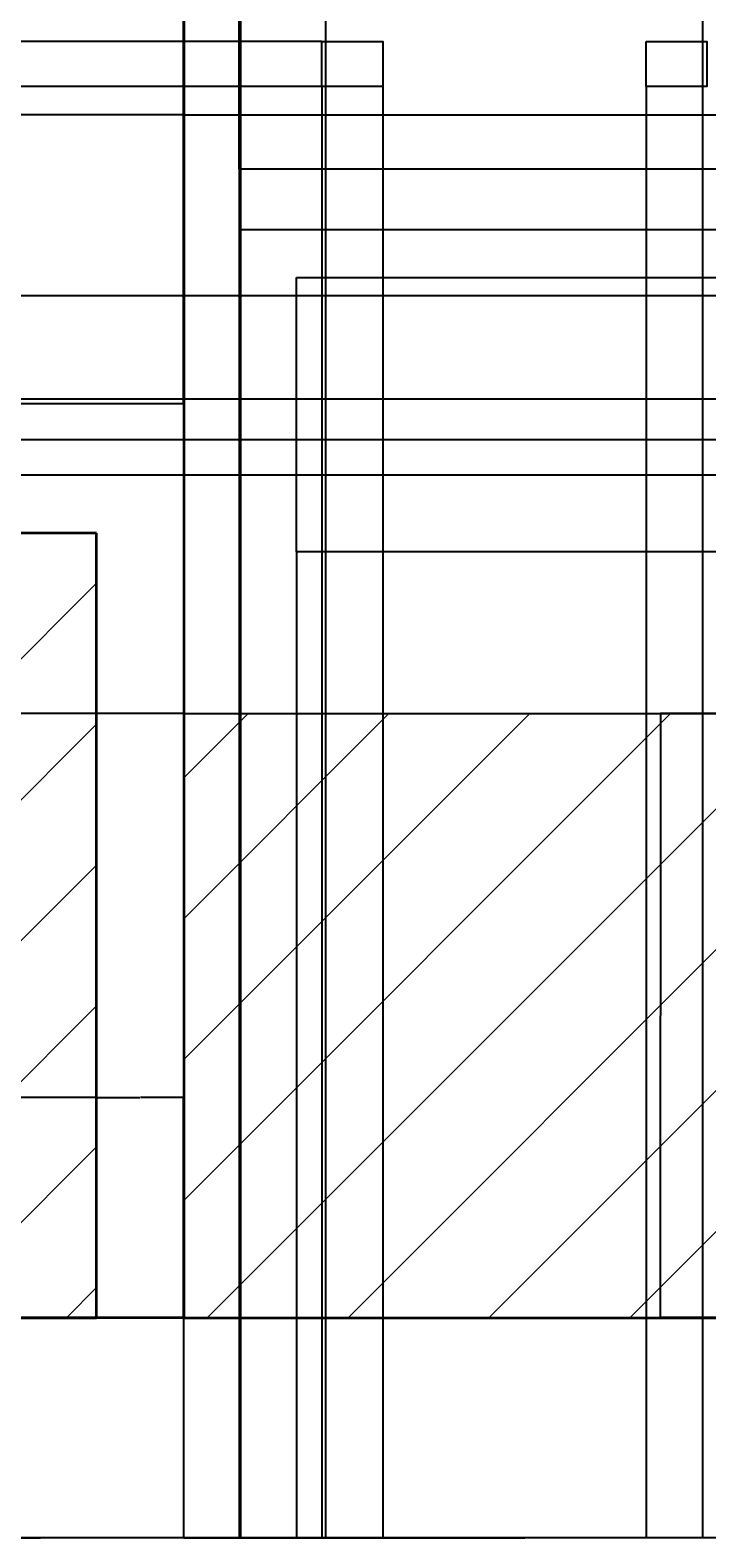
# Model space of a CAD drawing. Units: millimetres. Extents: x 2212 to 7718, y 1114 to 4219.
# Tile 3 of 5: x 5689 to 6466, y 1114 to 2844. Entities that reach past the tile are written whole.
import ezdxf

# ---------------------------------------------------------------- set-up
doc = ezdxf.new("R2010")
doc.units = ezdxf.units.MM
for name, color, linetype, lineweight in [('A-ANNO-DIMS', 2, 'Continuous', 18), ('A-ELEV-PATT', 8, 'Continuous', 13), ('A-EQPM', 4, 'Continuous', 25), ('A-FURN', 7, 'Continuous', 35), ('A-FURN-CTOP', 6, 'Continuous', 25)]:
    doc.layers.add(name, color=color, linetype=linetype, lineweight=lineweight)
doc.styles.get("Standard").update_dxf_attribs({"font": 'arial.ttf'})
doc.dimstyles.get("Standard").update_dxf_attribs({"dimtxt": 0.18, "dimasz": 0.18, "dimexe": 0.18, "dimexo": 0.0625, "dimgap": 0.09, "dimtad": 0, "dimtih": 1, "dimtoh": 1, "dimdec": 4, "dimzin": 0, "dimdsep": 46, "dimtxsty": 'Standard', "dimcen": 0.09, "dimadec": 0, "dimazin": 0, "dimtfac": 1, "dimtdec": 4, "dimtofl": 0, "dimtmove": 0, "dimatfit": 3, "dimfxl": 1, "dimtolj": 1, "dimtzin": 0, "dimarcsym": 0})

# ---------------------------------------------------------------- blocks, each defined once
blk = doc.blocks.new('*D16')
at = {"layer": 'A-ANNO-DIMS', "color": 0, "lineweight": -2, "transparency": 16777216}
for p, q in [((4965.1, 1366.2), (4965.1, 1618.9)), ((4965.3, 1618.7), (5364.9, 1618.7)), ((5765, 1618.7), (5365.4, 1618.7)), ((5765.1, 1366.2), (5765.1, 1618.9))]:
    blk.add_line(p, q, dxfattribs=at)
at = {"layer": 'A-ANNO-DIMS', "color": 0, "transparency": 16777216}
for points in [[(4965.3, 1618.7), (4965.3, 1618.7), (4965.1, 1618.7)], [(5765, 1618.7), (5765, 1618.7), (5765.1, 1618.7)]]:
    blk.add_solid(points, dxfattribs=at)
at = {"layer": 'Defpoints', "color": 0, "transparency": 16777216}
for p in [(5765.1, 1618.7), (4965.1, 1366.2), (5765.1, 1366.2)]:
    blk.add_point(p, dxfattribs=at)
at = {"layer": 'A-ANNO-DIMS', "color": 0, "transparency": 16777216, "insert": (5365.1, 1618.7), "char_height": 0.18, "attachment_point": 5}
blk.add_mtext('\\A1;800', dxfattribs=at)
blk = doc.blocks.new('*D17')
at = {"layer": 'A-ANNO-DIMS', "color": 0, "lineweight": -2, "transparency": 16777216}
for p, q in [((5765.1, 1366.2), (5765.1, 1618.9)), ((5765.3, 1618.7), (5814.9, 1618.7)), ((5865, 1618.7), (5815.4, 1618.7)), ((5865.1, 1366.2), (5865.1, 1618.9))]:
    blk.add_line(p, q, dxfattribs=at)
at = {"layer": 'A-ANNO-DIMS', "color": 0, "transparency": 16777216}
for points in [[(5765.3, 1618.7), (5765.3, 1618.7), (5765.1, 1618.7)], [(5865, 1618.7), (5865, 1618.7), (5865.1, 1618.7)]]:
    blk.add_solid(points, dxfattribs=at)
at = {"layer": 'Defpoints', "color": 0, "transparency": 16777216}
for p in [(5865.1, 1618.7), (5765.1, 1366.2), (5865.1, 1366.2)]:
    blk.add_point(p, dxfattribs=at)
at = {"layer": 'A-ANNO-DIMS', "color": 0, "transparency": 16777216, "insert": (5815.1, 1618.7), "char_height": 0.18, "attachment_point": 5}
blk.add_mtext('\\A1;100', dxfattribs=at)
blk = doc.blocks.new('*D18')
at = {"layer": 'A-ANNO-DIMS', "color": 0, "lineweight": -2, "transparency": 16777216}
for p, q in [((2465.1, 1366.1), (2465.1, 1113.5)), ((7465.1, 1366.1), (7465.1, 1113.5)), ((2465.3, 1113.7), (4964.8, 1113.7)), ((7465, 1113.7), (4965.5, 1113.7))]:
    blk.add_line(p, q, dxfattribs=at)
at = {"layer": 'A-ANNO-DIMS', "color": 0, "transparency": 16777216}
for points in [[(2465.3, 1113.7), (2465.3, 1113.7), (2465.1, 1113.7)], [(7465, 1113.7), (7465, 1113.7), (7465.1, 1113.7)]]:
    blk.add_solid(points, dxfattribs=at)
at = {"layer": 'Defpoints', "color": 0, "transparency": 16777216}
for p in [(2465.1, 1366.2), (7465.1, 1366.2), (7465.1, 1113.7)]:
    blk.add_point(p, dxfattribs=at)
at = {"layer": 'A-ANNO-DIMS', "color": 0, "transparency": 16777216, "insert": (4965.1, 1113.7), "char_height": 0.18, "attachment_point": 5}
blk.add_mtext('\\A1;5000', dxfattribs=at)
blk = doc.blocks.new('*D26')
at = {"layer": 'A-ANNO-DIMS', "color": 0, "lineweight": -2, "transparency": 16777216}
for p, q in [((6665.1, 2059.6), (6412.5, 2059.6)), ((6412.6, 2059.4), (6412.6, 1713.1)), ((6412.6, 1366.4), (6412.6, 1712.7)), ((6665.1, 1366.2), (6412.5, 1366.2))]:
    blk.add_line(p, q, dxfattribs=at)
at = {"layer": 'A-ANNO-DIMS', "color": 0, "transparency": 16777216}
for points in [[(6412.6, 2059.4), (6412.7, 2059.4), (6412.6, 2059.6)], [(6412.6, 1366.4), (6412.7, 1366.4), (6412.6, 1366.2)]]:
    blk.add_solid(points, dxfattribs=at)
at = {"layer": 'Defpoints', "color": 0, "transparency": 16777216}
for p in [(6412.6, 2059.6), (6665.1, 2059.6), (6665.1, 1366.2)]:
    blk.add_point(p, dxfattribs=at)
at = {"layer": 'A-ANNO-DIMS', "color": 0, "transparency": 16777216, "insert": (6412.6, 1712.9), "char_height": 0.18, "attachment_point": 5}
blk.add_mtext('\\A1;693.4', dxfattribs=at)
blk = doc.blocks.new('*D27')
at = {"layer": 'A-ANNO-DIMS', "color": 0, "lineweight": -2, "transparency": 16777216}
for p, q in [((5865.1, 2746.8), (2212.5, 2746.8)), ((2212.6, 2746.6), (2212.6, 2403.4)), ((2212.6, 2059.8), (2212.6, 2403)), ((5865.1, 2059.6), (2212.5, 2059.6))]:
    blk.add_line(p, q, dxfattribs=at)
at = {"layer": 'A-ANNO-DIMS', "color": 0, "transparency": 16777216}
for points in [[(2212.6, 2746.6), (2212.7, 2746.6), (2212.6, 2746.8)], [(2212.6, 2059.8), (2212.7, 2059.8), (2212.6, 2059.6)]]:
    blk.add_solid(points, dxfattribs=at)
at = {"layer": 'Defpoints', "color": 0, "transparency": 16777216}
for p in [(2212.6, 2746.8), (5865.1, 2746.8), (5865.1, 2059.6)]:
    blk.add_point(p, dxfattribs=at)
at = {"layer": 'A-ANNO-DIMS', "color": 0, "transparency": 16777216, "insert": (2212.6, 2403.2), "char_height": 0.18, "attachment_point": 5}
blk.add_mtext('\\A1;687.2', dxfattribs=at)
blk = doc.blocks.new('*D28')
at = {"layer": 'A-ANNO-DIMS', "color": 0, "lineweight": -2, "transparency": 16777216}
for p, q in [((5865.1, 2856.7), (2212.5, 2856.7)), ((2212.6, 2856.6), (2212.6, 2802)), ((2212.6, 2747), (2212.6, 2801.6)), ((5865.1, 2746.8), (2212.5, 2746.8))]:
    blk.add_line(p, q, dxfattribs=at)
at = {"layer": 'A-ANNO-DIMS', "color": 0, "transparency": 16777216}
for points in [[(2212.6, 2856.6), (2212.7, 2856.6), (2212.6, 2856.7)], [(2212.6, 2747), (2212.7, 2747), (2212.6, 2746.8)]]:
    blk.add_solid(points, dxfattribs=at)
at = {"layer": 'Defpoints', "color": 0, "transparency": 16777216}
for p in [(2212.6, 2856.7), (5865.1, 2856.7), (5865.1, 2746.8)]:
    blk.add_point(p, dxfattribs=at)
at = {"layer": 'A-ANNO-DIMS', "color": 0, "transparency": 16777216, "insert": (2212.6, 2801.8), "char_height": 0.18, "attachment_point": 5}
blk.add_mtext('\\A1;109.95', dxfattribs=at)
blk = doc.blocks.new('*D32')
at = {"layer": 'A-ANNO-DIMS', "color": 0, "lineweight": -2, "transparency": 16777216}
for p, q in [((5865.1, 3314.3), (5865.1, 1113.5)), ((5930.5, 3314.3), (5930.5, 1113.5)), ((5865.3, 1113.7), (5897.4, 1113.7)), ((5930.3, 1113.7), (5898.2, 1113.7))]:
    blk.add_line(p, q, dxfattribs=at)
at = {"layer": 'A-ANNO-DIMS', "color": 0, "transparency": 16777216}
for points in [[(5865.3, 1113.7), (5865.3, 1113.7), (5865.1, 1113.7)], [(5930.3, 1113.7), (5930.3, 1113.7), (5930.5, 1113.7)]]:
    blk.add_solid(points, dxfattribs=at)
at = {"layer": 'Defpoints', "color": 0, "transparency": 16777216}
for p in [(5865.1, 3314.4), (5930.5, 3314.4), (5930.5, 1113.7)]:
    blk.add_point(p, dxfattribs=at)
at = {"layer": 'A-ANNO-DIMS', "color": 0, "transparency": 16777216, "insert": (5897.8, 1113.7), "char_height": 0.18, "attachment_point": 5}
blk.add_mtext('\\A1;65.32', dxfattribs=at)
blk = doc.blocks.new('*D35')
at = {"layer": 'A-ANNO-DIMS', "color": 0, "lineweight": -2, "transparency": 16777216}
for p, q in [((6027.8, 2972.1), (6027.8, 1113.5)), ((6460.8, 2972.1), (6460.8, 1113.5)), ((6028, 1113.7), (6244, 1113.7)), ((6460.6, 1113.7), (6244.6, 1113.7))]:
    blk.add_line(p, q, dxfattribs=at)
at = {"layer": 'A-ANNO-DIMS', "color": 0, "transparency": 16777216}
for points in [[(6028, 1113.7), (6028, 1113.7), (6027.8, 1113.7)], [(6460.6, 1113.7), (6460.6, 1113.7), (6460.8, 1113.7)]]:
    blk.add_solid(points, dxfattribs=at)
at = {"layer": 'Defpoints', "color": 0, "transparency": 16777216}
for p in [(6027.8, 2972.2), (6460.8, 2972.2), (6460.8, 1113.7)]:
    blk.add_point(p, dxfattribs=at)
at = {"layer": 'A-ANNO-DIMS', "color": 0, "transparency": 16777216, "insert": (6244.3, 1113.7), "char_height": 0.18, "attachment_point": 5}
blk.add_mtext('\\A1;433', dxfattribs=at)
blk = doc.blocks.new('*D43')
at = {"layer": 'A-ANNO-DIMS', "color": 0, "lineweight": -2, "transparency": 16777216}
for p, q in [((6023.9, 2779.2), (6023.9, 1113.5)), ((6093.6, 2779.2), (6093.6, 1113.5)), ((6024.1, 1113.7), (6058.4, 1113.7)), ((6093.4, 1113.7), (6059.1, 1113.7))]:
    blk.add_line(p, q, dxfattribs=at)
at = {"layer": 'A-ANNO-DIMS', "color": 0, "transparency": 16777216}
for points in [[(6024.1, 1113.7), (6024.1, 1113.7), (6023.9, 1113.7)], [(6093.4, 1113.7), (6093.4, 1113.7), (6093.6, 1113.7)]]:
    blk.add_solid(points, dxfattribs=at)
at = {"layer": 'Defpoints', "color": 0, "transparency": 16777216}
for p in [(6023.9, 2779.3), (6093.6, 2779.3), (6093.6, 1113.7)]:
    blk.add_point(p, dxfattribs=at)
at = {"layer": 'A-ANNO-DIMS', "color": 0, "transparency": 16777216, "insert": (6058.7, 1113.7), "char_height": 0.18, "attachment_point": 5}
blk.add_mtext('\\A1;69.7', dxfattribs=at)
blk = doc.blocks.new('*D44')
at = {"layer": 'A-ANNO-DIMS', "color": 0, "lineweight": -2, "transparency": 16777216}
for p, q in [((6023.8, 2830.9), (2212.5, 2830.9)), ((2212.6, 2830.7), (2212.6, 2805.3)), ((2212.6, 2779.5), (2212.6, 2804.9)), ((6023.8, 2779.3), (2212.5, 2779.3))]:
    blk.add_line(p, q, dxfattribs=at)
at = {"layer": 'A-ANNO-DIMS', "color": 0, "transparency": 16777216}
for points in [[(2212.6, 2830.7), (2212.7, 2830.7), (2212.6, 2830.9)], [(2212.6, 2779.5), (2212.7, 2779.5), (2212.6, 2779.3)]]:
    blk.add_solid(points, dxfattribs=at)
at = {"layer": 'Defpoints', "color": 0, "transparency": 16777216}
for p in [(2212.6, 2830.9), (6023.9, 2830.9), (6023.9, 2779.3)]:
    blk.add_point(p, dxfattribs=at)
at = {"layer": 'A-ANNO-DIMS', "color": 0, "transparency": 16777216, "insert": (2212.6, 2805.1), "char_height": 0.18, "attachment_point": 5}
blk.add_mtext('\\A1;51.58', dxfattribs=at)
blk = doc.blocks.new('*D45')
at = {"layer": 'A-ANNO-DIMS', "color": 0, "lineweight": -2, "transparency": 16777216}
for p, q in [((6093.6, 2779.2), (6093.6, 1113.5)), ((6396, 2779.2), (6396, 1113.5)), ((6093.8, 1113.7), (6244.3, 1113.7)), ((6395.9, 1113.7), (6245.3, 1113.7))]:
    blk.add_line(p, q, dxfattribs=at)
at = {"layer": 'A-ANNO-DIMS', "color": 0, "transparency": 16777216}
for points in [[(6093.8, 1113.7), (6093.8, 1113.7), (6093.6, 1113.7)], [(6395.9, 1113.7), (6395.9, 1113.7), (6396, 1113.7)]]:
    blk.add_solid(points, dxfattribs=at)
at = {"layer": 'Defpoints', "color": 0, "transparency": 16777216}
for p in [(6093.6, 2779.3), (6396, 2779.3), (6396, 1113.7)]:
    blk.add_point(p, dxfattribs=at)
at = {"layer": 'A-ANNO-DIMS', "color": 0, "transparency": 16777216, "insert": (6244.8, 1113.7), "char_height": 0.18, "attachment_point": 5}
blk.add_mtext('\\A1;302.45', dxfattribs=at)
blk = doc.blocks.new('*D46')
at = {"layer": 'A-ANNO-DIMS', "color": 0, "lineweight": -2, "transparency": 16777216}
for p, q in [((6023.9, 2779.2), (6023.9, 1113.5)), ((5865.1, 2746.7), (5865.1, 1113.5)), ((5865.3, 1113.7), (5944.1, 1113.7)), ((6023.7, 1113.7), (5945, 1113.7))]:
    blk.add_line(p, q, dxfattribs=at)
at = {"layer": 'A-ANNO-DIMS', "color": 0, "transparency": 16777216}
for points in [[(5865.3, 1113.7), (5865.3, 1113.7), (5865.1, 1113.7)], [(6023.7, 1113.7), (6023.7, 1113.7), (6023.9, 1113.7)]]:
    blk.add_solid(points, dxfattribs=at)
at = {"layer": 'Defpoints', "color": 0, "transparency": 16777216}
for p in [(6023.9, 2779.3), (5865.1, 2746.8), (6023.9, 1113.7)]:
    blk.add_point(p, dxfattribs=at)
at = {"layer": 'A-ANNO-DIMS', "color": 0, "transparency": 16777216, "insert": (5944.5, 1113.7), "char_height": 0.18, "attachment_point": 5}
blk.add_mtext('\\A1;158.75', dxfattribs=at)
blk = doc.blocks.new('*D48')
at = {"layer": 'A-ANNO-DIMS', "color": 0, "lineweight": -2, "transparency": 16777216}
for p, q in [((5929, 2614.5), (5929, 1113.5)), ((6585.5, 2614.5), (6585.5, 1113.5)), ((5929.2, 1113.7), (6256.9, 1113.7)), ((6585.3, 1113.7), (6257.7, 1113.7))]:
    blk.add_line(p, q, dxfattribs=at)
at = {"layer": 'A-ANNO-DIMS', "color": 0, "transparency": 16777216}
for points in [[(5929.2, 1113.7), (5929.2, 1113.7), (5929, 1113.7)], [(6585.3, 1113.7), (6585.3, 1113.7), (6585.5, 1113.7)]]:
    blk.add_solid(points, dxfattribs=at)
at = {"layer": 'Defpoints', "color": 0, "transparency": 16777216}
for p in [(5929, 2614.6), (6585.5, 2614.6), (6585.5, 1113.7)]:
    blk.add_point(p, dxfattribs=at)
at = {"layer": 'A-ANNO-DIMS', "color": 0, "transparency": 16777216, "insert": (6257.3, 1113.7), "char_height": 0.18, "attachment_point": 5}
blk.add_mtext('\\A1;656.5', dxfattribs=at)
blk = doc.blocks.new('*D50')
at = {"layer": 'A-ANNO-DIMS', "color": 0, "lineweight": -2, "transparency": 16777216}
for p, q in [((5865.1, 2746.9), (5865.1, 4218.9)), ((5865.3, 4218.7), (5896.7, 4218.7)), ((5928.9, 4218.7), (5897.5, 4218.7)), ((5929, 2684.6), (5929, 4218.9))]:
    blk.add_line(p, q, dxfattribs=at)
at = {"layer": 'A-ANNO-DIMS', "color": 0, "transparency": 16777216}
for points in [[(5865.3, 4218.7), (5865.3, 4218.7), (5865.1, 4218.7)], [(5928.9, 4218.7), (5928.9, 4218.7), (5929, 4218.7)]]:
    blk.add_solid(points, dxfattribs=at)
at = {"layer": 'Defpoints', "color": 0, "transparency": 16777216}
for p in [(5929, 4218.7), (5865.1, 2746.8), (5929, 2684.5)]:
    blk.add_point(p, dxfattribs=at)
at = {"layer": 'A-ANNO-DIMS', "color": 0, "transparency": 16777216, "insert": (5897.1, 4218.7), "char_height": 0.18, "attachment_point": 5}
blk.add_mtext('\\A1;63.91', dxfattribs=at)
blk = doc.blocks.new('*D52')
at = {"layer": 'A-ANNO-DIMS', "color": 0, "lineweight": -2, "transparency": 16777216}
for p, q in [((5994.7, 2245), (5994.7, 1113.5)), ((6495.8, 2245), (6495.8, 1113.5)), ((5994.9, 1113.7), (6244.9, 1113.7)), ((6495.6, 1113.7), (6245.6, 1113.7))]:
    blk.add_line(p, q, dxfattribs=at)
at = {"layer": 'A-ANNO-DIMS', "color": 0, "transparency": 16777216}
for points in [[(5994.9, 1113.7), (5994.9, 1113.7), (5994.7, 1113.7)], [(6495.6, 1113.7), (6495.6, 1113.7), (6495.8, 1113.7)]]:
    blk.add_solid(points, dxfattribs=at)
at = {"layer": 'Defpoints', "color": 0, "transparency": 16777216}
for p in [(5994.7, 2245.1), (6495.8, 2245.1), (6495.8, 1113.7)]:
    blk.add_point(p, dxfattribs=at)
at = {"layer": 'A-ANNO-DIMS', "color": 0, "transparency": 16777216, "insert": (6245.3, 1113.7), "char_height": 0.18, "attachment_point": 5}
blk.add_mtext('\\A1;501.1', dxfattribs=at)
blk = doc.blocks.new('*D54')
at = {"layer": 'A-ANNO-DIMS', "color": 0, "lineweight": -2, "transparency": 16777216}
for p, q in [((5994.7, 2245), (5994.7, 1113.5)), ((5865.1, 2059.5), (5865.1, 1113.5)), ((5865.3, 1113.7), (5929.5, 1113.7)), ((5994.5, 1113.7), (5930.4, 1113.7))]:
    blk.add_line(p, q, dxfattribs=at)
at = {"layer": 'A-ANNO-DIMS', "color": 0, "transparency": 16777216}
for points in [[(5865.3, 1113.7), (5865.3, 1113.7), (5865.1, 1113.7)], [(5994.5, 1113.7), (5994.5, 1113.7), (5994.7, 1113.7)]]:
    blk.add_solid(points, dxfattribs=at)
at = {"layer": 'Defpoints', "color": 0, "transparency": 16777216}
for p in [(5994.7, 2245.1), (5865.1, 2059.6), (5994.7, 1113.7)]:
    blk.add_point(p, dxfattribs=at)
at = {"layer": 'A-ANNO-DIMS', "color": 0, "transparency": 16777216, "insert": (5929.9, 1113.7), "char_height": 0.18, "attachment_point": 5}
blk.add_mtext('\\A1;129.56', dxfattribs=at)
blk = doc.blocks.new('*D62')
at = {"layer": 'A-ANNO-DIMS', "color": 0, "lineweight": -2, "transparency": 16777216}
for p, q in [((5537.5, 2333.3), (5537.5, 1113.5)), ((5865.1, 2333.3), (5865.1, 1113.5)), ((5537.7, 1113.7), (5700.8, 1113.7)), ((5865, 1113.7), (5701.8, 1113.7))]:
    blk.add_line(p, q, dxfattribs=at)
at = {"layer": 'A-ANNO-DIMS', "color": 0, "transparency": 16777216}
for points in [[(5537.7, 1113.7), (5537.7, 1113.7), (5537.5, 1113.7)], [(5865, 1113.7), (5865, 1113.7), (5865.1, 1113.7)]]:
    blk.add_solid(points, dxfattribs=at)
at = {"layer": 'Defpoints', "color": 0, "transparency": 16777216}
for p in [(5537.5, 2333.4), (5865.1, 2333.4), (5865.1, 1113.7)]:
    blk.add_point(p, dxfattribs=at)
at = {"layer": 'A-ANNO-DIMS', "color": 0, "transparency": 16777216, "insert": (5701.3, 1113.7), "char_height": 0.18, "attachment_point": 5}
blk.add_mtext('\\A1;327.66', dxfattribs=at)
blk = doc.blocks.new('*D71')
at = {"layer": 'A-ANNO-DIMS', "color": 0, "lineweight": -2, "transparency": 16777216}
for p, q in [((5608.2, 2374.1), (7717.8, 2374.1)), ((7717.6, 2373.9), (7717.6, 2353.9)), ((7717.6, 2333.5), (7717.6, 2353.5)), ((5537.5, 2333.4), (7717.8, 2333.4))]:
    blk.add_line(p, q, dxfattribs=at)
at = {"layer": 'A-ANNO-DIMS', "color": 0, "transparency": 16777216}
for points in [[(7717.6, 2373.9), (7717.7, 2373.9), (7717.6, 2374.1)], [(7717.6, 2333.5), (7717.7, 2333.5), (7717.6, 2333.4)]]:
    blk.add_solid(points, dxfattribs=at)
at = {"layer": 'Defpoints', "color": 0, "transparency": 16777216}
for p in [(5608.2, 2374.1), (7717.6, 2374.1), (5537.5, 2333.4)]:
    blk.add_point(p, dxfattribs=at)
at = {"layer": 'A-ANNO-DIMS', "color": 0, "transparency": 16777216, "insert": (7717.6, 2353.7), "char_height": 0.18, "attachment_point": 5}
blk.add_mtext('\\A1;40.726', dxfattribs=at)
blk = doc.blocks.new('*D73')
at = {"layer": 'A-ANNO-DIMS', "color": 0, "lineweight": -2, "transparency": 16777216}
for p, q in [((5284.8, 2539.3), (7717.8, 2539.3)), ((7717.6, 2539.1), (7717.6, 2480.2)), ((7717.6, 2420.9), (7717.6, 2479.8)), ((5329.4, 2420.7), (7717.8, 2420.7))]:
    blk.add_line(p, q, dxfattribs=at)
at = {"layer": 'A-ANNO-DIMS', "color": 0, "transparency": 16777216}
for points in [[(7717.6, 2539.1), (7717.7, 2539.1), (7717.6, 2539.3)], [(7717.6, 2420.9), (7717.7, 2420.9), (7717.6, 2420.7)]]:
    blk.add_solid(points, dxfattribs=at)
at = {"layer": 'Defpoints', "color": 0, "transparency": 16777216}
for p in [(5284.8, 2539.3), (7717.6, 2539.3), (5329.3, 2420.7)]:
    blk.add_point(p, dxfattribs=at)
at = {"layer": 'A-ANNO-DIMS', "color": 0, "transparency": 16777216, "insert": (7717.6, 2480), "char_height": 0.18, "attachment_point": 5}
blk.add_mtext('\\A1;118.60', dxfattribs=at)
blk = doc.blocks.new('*D74')
at = {"layer": 'A-ANNO-DIMS', "color": 0, "lineweight": -2, "transparency": 16777216}
for p, q in [((5335.2, 2434.9), (5335.2, 4218.9)), ((5335.4, 4218.7), (5599.7, 4218.7)), ((5865, 4218.7), (5600.6, 4218.7)), ((5865.1, 2414.9), (5865.1, 4218.9))]:
    blk.add_line(p, q, dxfattribs=at)
at = {"layer": 'A-ANNO-DIMS', "color": 0, "transparency": 16777216}
for points in [[(5335.4, 4218.7), (5335.4, 4218.7), (5335.2, 4218.7)], [(5865, 4218.7), (5865, 4218.7), (5865.1, 4218.7)]]:
    blk.add_solid(points, dxfattribs=at)
at = {"layer": 'Defpoints', "color": 0, "transparency": 16777216}
for p in [(5865.1, 4218.7), (5335.2, 2434.8), (5865.1, 2414.8)]:
    blk.add_point(p, dxfattribs=at)
at = {"layer": 'A-ANNO-DIMS', "color": 0, "transparency": 16777216, "insert": (5600.2, 4218.7), "char_height": 0.18, "attachment_point": 5}
blk.add_mtext('\\A1;529.94', dxfattribs=at)

msp = doc.modelspace()

# ---------------------------------------------------------------- hatches: boundary and pattern name
at = {"layer": 'A-ELEV-PATT'}
h = msp.add_hatch(dxfattribs=at)
h.set_pattern_fill('ANSI31', color=256, scale=36)
h.paths.add_polyline_path([(3153.454, 3966.1829), (2465.1412, 3966.1829), (2465.1412, 3121.3339), (3153.454, 3121.3339)])
h.paths.add_polyline_path([(3659.2976, 3966.1829), (3153.454, 3966.1829), (3153.454, 3121.3339), (3659.2976, 3121.3339)])
h.paths.add_polyline_path([(4165.1412, 3966.1829), (3659.2976, 3966.1829), (3659.2976, 3121.3339), (4165.1412, 3121.3339)])
h.paths.add_polyline_path([(3365.1412, 2266.3983), (2465.1412, 2266.3983), (2465.1412, 1366.1829), (3365.1412, 1366.1829)])
h.paths.add_polyline_path([(4165.1412, 2266.3983), (3365.1412, 2266.3983), (3365.1412, 1366.1829), (4165.1412, 1366.1829)])
h.paths.add_polyline_path([(4965.1412, 2266.3983), (4165.1412, 2266.3983), (4165.1412, 1366.1829), (4965.1412, 1366.1829)])
h.paths.add_polyline_path([(5765.1412, 2266.3983), (4965.1412, 2266.3983), (4965.1412, 1366.1829), (5765.1412, 1366.1829)])
h.paths.add_polyline_path([(6665.1412, 2059.6125), (5865.1412, 2059.6125), (5865.1412, 1366.1829), (6665.1412, 1366.1829)])
h.paths.add_polyline_path([(7465.1412, 2266.3983), (7065.1412, 2266.3983), (7065.1412, 1366.1829), (7465.1412, 1366.1829)])
h.paths.add_polyline_path([(7065.1412, 2266.3983), (6665.1412, 2266.3983), (6665.1412, 1366.1829), (7065.1412, 1366.1829)])
h.paths.add_polyline_path([(7465.1412, 3966.1829), (7065.1412, 3966.1829), (7065.1412, 2266.3983), (7465.1412, 2266.3983)])
h.paths.add_polyline_path([(7065.1412, 3966.1829), (6665.1412, 3966.1829), (6665.1412, 2266.3983), (7065.1412, 2266.3983)])
h.paths.add_polyline_path([(6665.1412, 3966.1829), (6027.7806, 3966.1829), (6027.7806, 3314.3715), (6665.1412, 3314.3715)])
h.paths.add_polyline_path([(5245.7331, 3966.1829), (4821.5849, 3966.1829), (4821.5849, 3216.3983), (4356.7186, 3216.3983), (4356.7186, 3121.3339), (5503.6152, 3121.3339), (5720.779, 3121.3339), (5720.779, 3216.3983), (5245.7331, 3216.3983)])

# ---------------------------------------------------------------- linework, layer by layer
at = {"layer": 'A-EQPM'}
for p, q in [((5865.1412, 2746.7954), (6665.1412, 2746.7954)), ((5865.1412, 2059.6125), (6665.1412, 2059.6125))]:
    msp.add_line(p, q, dxfattribs=at)
for points in [[(6023.8866, 2830.8799), (6093.5841, 2830.8799), (6093.5841, 2779.2966), (6023.8866, 2779.2966)], [(6396.0365, 2830.8799), (6465.7339, 2830.8799), (6465.7339, 2779.2966), (6396.0365, 2779.2966)], [(5929.0495, 2684.5306), (6585.5248, 2684.5306), (6585.5248, 2614.5667), (5929.0495, 2614.5667)], [(5994.697, 2559.9075), (6495.8065, 2559.9075), (6495.8065, 2245.0701), (5994.697, 2245.0701)]]:
    msp.add_lwpolyline(points, close=True, dxfattribs=at)
at = {"layer": 'A-FURN'}
for p, q in [((5865.1412, 3966.1829), (5865.1412, 1366.1829)), ((5765.1412, 2266.3983), (2465.1412, 2266.3983)), ((5765.1412, 1366.1829), (5765.1412, 2266.3983)), ((5865.1412, 1366.1829), (2465.1412, 1366.1829)), ((4965.1412, 1366.1829), (5765.1412, 1366.1829)), ((5865.1412, 1366.1829), (6665.1412, 1366.1829))]:
    msp.add_line(p, q, dxfattribs=at)
at = {"layer": 'A-FURN-CTOP'}
for p, q in [((5865.1412, 2414.8193), (2465.1412, 2414.8193)), ((2465.1412, 2333.3682), (5865.1412, 2333.3682))]:
    msp.add_line(p, q, dxfattribs=at)

# ---------------------------------------------------------------- dimensions: what is measured, and where the dimension line sits
at = {"layer": 'A-ANNO-DIMS'}
for base, p1, p2, override, picture, middle in [((5865.1412, 4218.6829), (5335.1967, 2434.8193), (5865.1412, 2414.8193), {"dimdec": 2, "dimlfac": 1, "dimrnd": 0, "dimzin": 0, "dimdsep": 46, "dimlunit": 2}, '*D74', (5600.1689, 4218.6829)), ((5929.0495, 4218.6829), (5865.1412, 2746.7954), (5929.0495, 2684.5306), {"dimdec": 2, "dimlfac": 1, "dimrnd": 0, "dimzin": 0, "dimdsep": 46, "dimlunit": 2}, '*D50', (5897.0953, 4218.6829)), ((5930.461, 1113.6829), (5865.1412, 3314.3715), (5930.461, 3314.3715), {"dimdec": 2, "dimlfac": 1, "dimrnd": 0, "dimzin": 0, "dimdsep": 46, "dimlunit": 2}, '*D32', (5897.8011, 1113.6829)), ((6460.8234, 1113.6829), (6027.7806, 2972.1846), (6460.8234, 2972.1846), {"dimdec": 0, "dimlfac": 1, "dimrnd": 0, "dimzin": 0, "dimdsep": 46, "dimlunit": 2}, '*D35', (6244.302, 1113.6829)), ((6023.8866, 1113.6829), (5865.1412, 2746.7954), (6023.8866, 2779.2966), {"dimdec": 2, "dimlfac": 1, "dimrnd": 0, "dimzin": 0, "dimdsep": 46, "dimlunit": 2}, '*D46', (5944.5139, 1113.6829)), ((6093.5841, 1113.6829), (6023.8866, 2779.2966), (6093.5841, 2779.2966), {"dimdec": 1, "dimlfac": 1, "dimrnd": 0, "dimzin": 0, "dimdsep": 46, "dimlunit": 2}, '*D43', (6058.7354, 1113.6829)), ((6396.0365, 1113.6829), (6093.5841, 2779.2966), (6396.0365, 2779.2966), {"dimdec": 2, "dimlfac": 1, "dimrnd": 0, "dimzin": 0, "dimdsep": 46, "dimlunit": 2}, '*D45', (6244.8103, 1113.6829)), ((6585.5248, 1113.6829), (5929.0495, 2614.5667), (6585.5248, 2614.5667), {"dimdec": 1, "dimlfac": 1, "dimrnd": 0, "dimzin": 0, "dimdsep": 46, "dimlunit": 2}, '*D48', (6257.2872, 1113.6829)), ((5865.1412, 1113.6829), (5537.4832, 2333.3682), (5865.1412, 2333.3682), {"dimdec": 2, "dimlfac": 1, "dimrnd": 0, "dimzin": 0, "dimdsep": 46, "dimlunit": 2}, '*D62', (5701.3122, 1113.6829)), ((5994.697, 1113.6829), (5865.1412, 2059.6125), (5994.697, 2245.0701), {"dimdec": 2, "dimlfac": 1, "dimrnd": 0, "dimzin": 0, "dimdsep": 46, "dimlunit": 2}, '*D54', (5929.9191, 1113.6829)), ((6495.8065, 1113.6829), (5994.697, 2245.0701), (6495.8065, 2245.0701), {"dimdec": 1, "dimlfac": 1, "dimrnd": 0, "dimzin": 0, "dimdsep": 46, "dimlunit": 2}, '*D52', (6245.2518, 1113.6829)), ((5765.1412, 1618.6829), (4965.1412, 1366.1829), (5765.1412, 1366.1829), {"dimdec": 0, "dimlfac": 1, "dimrnd": 0, "dimzin": 0, "dimdsep": 46, "dimlunit": 2}, '*D16', (5365.1412, 1618.6829)), ((5865.1412, 1618.6829), (5765.1412, 1366.1829), (5865.1412, 1366.1829), {"dimdec": 0, "dimlfac": 1, "dimrnd": 0, "dimzin": 0, "dimdsep": 46, "dimlunit": 2}, '*D17', (5815.1412, 1618.6829)), ((7465.1412, 1113.6829), (2465.1412, 1366.1829), (7465.1412, 1366.1829), {"dimdec": 0, "dimlfac": 1, "dimrnd": 0, "dimzin": 0, "dimdsep": 46, "dimlunit": 2}, '*D18', (4965.1412, 1113.6829))]:
    dim = msp.add_linear_dim(base=base, p1=p1, p2=p2, dimstyle='Standard', override=override, dxfattribs=at)
    dim.commit()
    dim.dimension.update_dxf_attribs({"geometry": picture, "text_midpoint": middle})
for base, p1, p2, override, picture, middle in [((2212.6412, 2856.7409), (5865.1412, 2746.7954), (5865.1412, 2856.7409), {"dimdec": 2, "dimlfac": 1, "dimrnd": 0, "dimzin": 0, "dimdsep": 46, "dimlunit": 2}, '*D28', (2212.6412, 2801.7682)), ((2212.6412, 2830.8799), (6023.8866, 2779.2966), (6023.8866, 2830.8799), {"dimdec": 2, "dimlfac": 1, "dimrnd": 0, "dimzin": 0, "dimdsep": 46, "dimlunit": 2}, '*D44', (2212.6412, 2805.0882)), ((2212.6412, 2746.7954), (5865.1412, 2059.6125), (5865.1412, 2746.7954), {"dimdec": 1, "dimlfac": 1, "dimrnd": 0, "dimzin": 0, "dimdsep": 46, "dimlunit": 2}, '*D27', (2212.6412, 2403.204)), ((7717.6412, 2539.2808), (5329.3388, 2420.6771), (5284.7847, 2539.2808), {"dimdec": 2, "dimlfac": 1, "dimrnd": 0, "dimzin": 0, "dimdsep": 46, "dimlunit": 2}, '*D73', (7717.6412, 2479.979)), ((7717.64116, 2374.09375), (5537.48322, 2333.36822), (5608.17143, 2374.09375), {"dimdec": 3, "dimlfac": 1, "dimrnd": 0, "dimzin": 0, "dimdsep": 46, "dimlunit": 2}, '*D71', (7717.64116, 2353.73098)), ((6412.6412, 2059.6125), (6665.1412, 1366.1829), (6665.1412, 2059.6125), {"dimdec": 1, "dimlfac": 1, "dimrnd": 0, "dimzin": 0, "dimdsep": 46, "dimlunit": 2}, '*D26', (6412.6412, 1712.8977))]:
    dim = msp.add_linear_dim(base=base, p1=p1, p2=p2, angle=90, dimstyle='Standard', override=override, dxfattribs=at)
    dim.commit()
    dim.dimension.update_dxf_attribs({"geometry": picture, "text_midpoint": middle})

doc.saveas('drawing.dxf')
